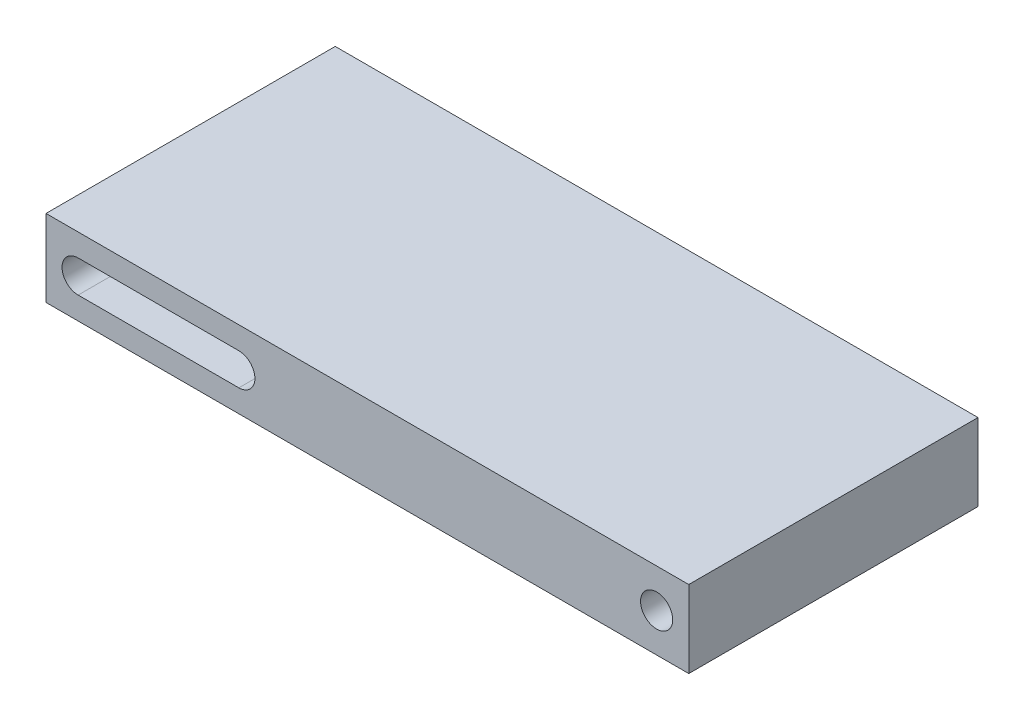
ISO-10303-21;
HEADER;
FILE_DESCRIPTION(('STEP AP214'),'2;1');
FILE_NAME('part.step','',(''),(''),'','','');
FILE_SCHEMA(('AUTOMOTIVE_DESIGN { 1 0 10303 214 1 1 1 1 }'));
ENDSEC;
DATA;
#1=APPLICATION_CONTEXT('core data for automotive mechanical design processes');
#2=APPLICATION_PROTOCOL_DEFINITION('international standard','automotive_design',2000,#1);
#3=PRODUCT_CONTEXT('',#1,'mechanical');
#4=PRODUCT('Part','Part','',(#3));
#5=PRODUCT_RELATED_PRODUCT_CATEGORY('part','',(#4));
#6=PRODUCT_DEFINITION_FORMATION('','',#4);
#7=PRODUCT_DEFINITION_CONTEXT('part definition',#1,'design');
#8=PRODUCT_DEFINITION('design','',#6,#7);
#9=PRODUCT_DEFINITION_SHAPE('','',#8);
#10=(LENGTH_UNIT() NAMED_UNIT(*) SI_UNIT(.MILLI.,.METRE.));
#11=(NAMED_UNIT(*) PLANE_ANGLE_UNIT() SI_UNIT($,.RADIAN.));
#12=(NAMED_UNIT(*) SI_UNIT($,.STERADIAN.) SOLID_ANGLE_UNIT());
#13=UNCERTAINTY_MEASURE_WITH_UNIT(LENGTH_MEASURE(1.E-05),#10,'distance_accuracy_value','');
#14=(GEOMETRIC_REPRESENTATION_CONTEXT(3) GLOBAL_UNCERTAINTY_ASSIGNED_CONTEXT((#13)) GLOBAL_UNIT_ASSIGNED_CONTEXT((#10,
#11,#12)) REPRESENTATION_CONTEXT('',''));
#15=CARTESIAN_POINT('',(0.,0.,0.));
#16=DIRECTION('',(0.,0.,1.));
#17=DIRECTION('',(1.,0.,0.));
#18=AXIS2_PLACEMENT_3D('',#15,#16,#17);
#19=CARTESIAN_POINT('',(50.,6.,22.5));
#20=DIRECTION('',(-1.,0.,0.));
#21=DIRECTION('',(0.,0.,1.));
#22=AXIS2_PLACEMENT_3D('',#19,#20,#21);
#23=PLANE('',#22);
#24=DIRECTION('',(0.,1.,0.));
#25=VECTOR('',#24,1.);
#26=CARTESIAN_POINT('',(50.,6.,-22.5));
#27=LINE('',#26,#25);
#28=CARTESIAN_POINT('',(50.,-6.,-22.5));
#29=VERTEX_POINT('',#28);
#30=CARTESIAN_POINT('',(50.,6.,-22.5));
#31=VERTEX_POINT('',#30);
#32=EDGE_CURVE('E116',#29,#31,#27,.T.);
#33=ORIENTED_EDGE('',*,*,#32,.T.);
#34=DIRECTION('',(0.,0.,-1.));
#35=VECTOR('',#34,1.);
#36=CARTESIAN_POINT('',(50.,6.,22.5));
#37=LINE('',#36,#35);
#38=CARTESIAN_POINT('',(50.,6.,22.5));
#39=VERTEX_POINT('',#38);
#40=EDGE_CURVE('E11',#39,#31,#37,.T.);
#41=ORIENTED_EDGE('',*,*,#40,.F.);
#42=DIRECTION('',(0.,1.,0.));
#43=VECTOR('',#42,1.);
#44=CARTESIAN_POINT('',(50.,6.,22.5));
#45=LINE('',#44,#43);
#46=CARTESIAN_POINT('',(50.,-6.,22.5));
#47=VERTEX_POINT('',#46);
#48=EDGE_CURVE('E148',#47,#39,#45,.T.);
#49=ORIENTED_EDGE('',*,*,#48,.F.);
#50=DIRECTION('',(0.,0.,-1.));
#51=VECTOR('',#50,1.);
#52=CARTESIAN_POINT('',(50.,-6.,22.5));
#53=LINE('',#52,#51);
#54=EDGE_CURVE('E156',#47,#29,#53,.T.);
#55=ORIENTED_EDGE('',*,*,#54,.T.);
#56=EDGE_LOOP('',(#33,#41,#49,#55));
#57=FACE_BOUND('',#56,.T.);
#58=ADVANCED_FACE('F39',(#57),#23,.F.);
#59=CARTESIAN_POINT('',(-50.,6.,22.5));
#60=DIRECTION('',(0.,-1.,0.));
#61=DIRECTION('',(0.,0.,-1.));
#62=AXIS2_PLACEMENT_3D('',#59,#60,#61);
#63=PLANE('',#62);
#64=DIRECTION('',(-1.,0.,0.));
#65=VECTOR('',#64,1.);
#66=CARTESIAN_POINT('',(-50.,6.,-22.5));
#67=LINE('',#66,#65);
#68=CARTESIAN_POINT('',(-50.,6.,-22.5));
#69=VERTEX_POINT('',#68);
#70=EDGE_CURVE('E157',#31,#69,#67,.T.);
#71=ORIENTED_EDGE('',*,*,#70,.T.);
#72=DIRECTION('',(0.,0.,-1.));
#73=VECTOR('',#72,1.);
#74=CARTESIAN_POINT('',(-50.,6.,22.5));
#75=LINE('',#74,#73);
#76=CARTESIAN_POINT('',(-50.,6.,22.5));
#77=VERTEX_POINT('',#76);
#78=EDGE_CURVE('E46',#77,#69,#75,.T.);
#79=ORIENTED_EDGE('',*,*,#78,.F.);
#80=DIRECTION('',(-1.,0.,0.));
#81=VECTOR('',#80,1.);
#82=CARTESIAN_POINT('',(-50.,6.,22.5));
#83=LINE('',#82,#81);
#84=EDGE_CURVE('E149',#39,#77,#83,.T.);
#85=ORIENTED_EDGE('',*,*,#84,.F.);
#86=ORIENTED_EDGE('',*,*,#40,.T.);
#87=EDGE_LOOP('',(#71,#79,#85,#86));
#88=FACE_BOUND('',#87,.T.);
#89=ADVANCED_FACE('F190',(#88),#63,.F.);
#90=CARTESIAN_POINT('',(-50.,6.,22.5));
#91=DIRECTION('',(1.,0.,0.));
#92=DIRECTION('',(0.,0.,-1.));
#93=AXIS2_PLACEMENT_3D('',#90,#91,#92);
#94=PLANE('',#93);
#95=DIRECTION('',(0.,-1.,0.));
#96=VECTOR('',#95,1.);
#97=CARTESIAN_POINT('',(-50.,6.,-22.5));
#98=LINE('',#97,#96);
#99=CARTESIAN_POINT('',(-50.,-6.,-22.5));
#100=VERTEX_POINT('',#99);
#101=EDGE_CURVE('E161',#69,#100,#98,.T.);
#102=ORIENTED_EDGE('',*,*,#101,.T.);
#103=DIRECTION('',(0.,0.,-1.));
#104=VECTOR('',#103,1.);
#105=CARTESIAN_POINT('',(-50.,-6.,22.5));
#106=LINE('',#105,#104);
#107=CARTESIAN_POINT('',(-50.,-6.,22.5));
#108=VERTEX_POINT('',#107);
#109=EDGE_CURVE('E167',#108,#100,#106,.T.);
#110=ORIENTED_EDGE('',*,*,#109,.F.);
#111=DIRECTION('',(0.,-1.,0.));
#112=VECTOR('',#111,1.);
#113=CARTESIAN_POINT('',(-50.,6.,22.5));
#114=LINE('',#113,#112);
#115=EDGE_CURVE('E155',#77,#108,#114,.T.);
#116=ORIENTED_EDGE('',*,*,#115,.F.);
#117=ORIENTED_EDGE('',*,*,#78,.T.);
#118=EDGE_LOOP('',(#102,#110,#116,#117));
#119=FACE_BOUND('',#118,.T.);
#120=ADVANCED_FACE('F175',(#119),#94,.F.);
#121=CARTESIAN_POINT('',(-50.,-6.,22.5));
#122=DIRECTION('',(0.,1.,0.));
#123=DIRECTION('',(0.,0.,1.));
#124=AXIS2_PLACEMENT_3D('',#121,#122,#123);
#125=PLANE('',#124);
#126=DIRECTION('',(1.,0.,0.));
#127=VECTOR('',#126,1.);
#128=CARTESIAN_POINT('',(-50.,-6.,-22.5));
#129=LINE('',#128,#127);
#130=EDGE_CURVE('E147',#100,#29,#129,.T.);
#131=ORIENTED_EDGE('',*,*,#130,.T.);
#132=ORIENTED_EDGE('',*,*,#54,.F.);
#133=DIRECTION('',(1.,0.,0.));
#134=VECTOR('',#133,1.);
#135=CARTESIAN_POINT('',(-50.,-6.,22.5));
#136=LINE('',#135,#134);
#137=EDGE_CURVE('E152',#108,#47,#136,.T.);
#138=ORIENTED_EDGE('',*,*,#137,.F.);
#139=ORIENTED_EDGE('',*,*,#109,.T.);
#140=EDGE_LOOP('',(#131,#132,#138,#139));
#141=FACE_BOUND('',#140,.T.);
#142=ADVANCED_FACE('F182',(#141),#125,.F.);
#143=CARTESIAN_POINT('',(0.,0.,22.5));
#144=DIRECTION('',(0.,0.,1.));
#145=DIRECTION('',(1.,0.,0.));
#146=AXIS2_PLACEMENT_3D('',#143,#144,#145);
#147=PLANE('',#146);
#148=CARTESIAN_POINT('',(-45.,0.,22.5));
#149=DIRECTION('',(0.,0.,1.));
#150=DIRECTION('',(1.,0.,0.));
#151=AXIS2_PLACEMENT_3D('',#148,#149,#150);
#152=CIRCLE('',#151,2.5);
#153=CARTESIAN_POINT('',(-45.,2.5,22.5));
#154=VERTEX_POINT('',#153);
#155=CARTESIAN_POINT('',(-45.,-2.5,22.5));
#156=VERTEX_POINT('',#155);
#157=EDGE_CURVE('E52',#154,#156,#152,.T.);
#158=ORIENTED_EDGE('',*,*,#157,.F.);
#159=DIRECTION('',(-1.,0.,0.));
#160=VECTOR('',#159,1.);
#161=CARTESIAN_POINT('',(-45.,2.5,22.5));
#162=LINE('',#161,#160);
#163=CARTESIAN_POINT('',(-20.,2.5,22.5));
#164=VERTEX_POINT('',#163);
#165=EDGE_CURVE('E112',#164,#154,#162,.T.);
#166=ORIENTED_EDGE('',*,*,#165,.F.);
#167=CARTESIAN_POINT('',(-20.,0.,22.5));
#168=DIRECTION('',(0.,0.,1.));
#169=DIRECTION('',(1.,0.,0.));
#170=AXIS2_PLACEMENT_3D('',#167,#168,#169);
#171=CIRCLE('',#170,2.5);
#172=CARTESIAN_POINT('',(-20.,-2.5,22.5));
#173=VERTEX_POINT('',#172);
#174=EDGE_CURVE('E134',#173,#164,#171,.T.);
#175=ORIENTED_EDGE('',*,*,#174,.F.);
#176=DIRECTION('',(1.,0.,0.));
#177=VECTOR('',#176,1.);
#178=CARTESIAN_POINT('',(-45.,-2.5,22.5));
#179=LINE('',#178,#177);
#180=EDGE_CURVE('E124',#156,#173,#179,.T.);
#181=ORIENTED_EDGE('',*,*,#180,.F.);
#182=EDGE_LOOP('',(#158,#166,#175,#181));
#183=FACE_BOUND('',#182,.T.);
#184=CARTESIAN_POINT('',(45.,0.,22.5));
#185=DIRECTION('',(0.,0.,1.));
#186=DIRECTION('',(1.,0.,0.));
#187=AXIS2_PLACEMENT_3D('',#184,#185,#186);
#188=CIRCLE('',#187,2.5);
#189=CARTESIAN_POINT('',(47.5,0.,22.5));
#190=VERTEX_POINT('',#189);
#191=EDGE_CURVE('E139',#190,#190,#188,.T.);
#192=ORIENTED_EDGE('',*,*,#191,.F.);
#193=EDGE_LOOP('',(#192));
#194=FACE_BOUND('',#193,.T.);
#195=ORIENTED_EDGE('',*,*,#48,.T.);
#196=ORIENTED_EDGE('',*,*,#84,.T.);
#197=ORIENTED_EDGE('',*,*,#115,.T.);
#198=ORIENTED_EDGE('',*,*,#137,.T.);
#199=EDGE_LOOP('',(#195,#196,#197,#198));
#200=FACE_BOUND('',#199,.T.);
#201=ADVANCED_FACE('F186',(#183,#194,#200),#147,.T.);
#202=CARTESIAN_POINT('',(0.,0.,-22.5));
#203=DIRECTION('',(0.,0.,1.));
#204=DIRECTION('',(1.,0.,0.));
#205=AXIS2_PLACEMENT_3D('',#202,#203,#204);
#206=PLANE('',#205);
#207=DIRECTION('',(1.,0.,0.));
#208=VECTOR('',#207,1.);
#209=CARTESIAN_POINT('',(-45.,2.5,-22.5));
#210=LINE('',#209,#208);
#211=CARTESIAN_POINT('',(-45.,2.5,-22.5));
#212=VERTEX_POINT('',#211);
#213=CARTESIAN_POINT('',(-20.,2.5,-22.5));
#214=VERTEX_POINT('',#213);
#215=EDGE_CURVE('E122',#212,#214,#210,.T.);
#216=ORIENTED_EDGE('',*,*,#215,.F.);
#217=CARTESIAN_POINT('',(-45.,0.,-22.5));
#218=DIRECTION('',(0.,0.,1.));
#219=DIRECTION('',(1.,0.,0.));
#220=AXIS2_PLACEMENT_3D('',#217,#218,#219);
#221=CIRCLE('',#220,2.5);
#222=CARTESIAN_POINT('',(-45.,-2.5,-22.5));
#223=VERTEX_POINT('',#222);
#224=EDGE_CURVE('E104',#223,#212,#221,.F.);
#225=ORIENTED_EDGE('',*,*,#224,.F.);
#226=DIRECTION('',(-1.,0.,0.));
#227=VECTOR('',#226,1.);
#228=CARTESIAN_POINT('',(-45.,-2.5,-22.5));
#229=LINE('',#228,#227);
#230=CARTESIAN_POINT('',(-20.,-2.5,-22.5));
#231=VERTEX_POINT('',#230);
#232=EDGE_CURVE('E111',#231,#223,#229,.T.);
#233=ORIENTED_EDGE('',*,*,#232,.F.);
#234=CARTESIAN_POINT('',(-20.,0.,-22.5));
#235=DIRECTION('',(0.,0.,1.));
#236=DIRECTION('',(1.,0.,0.));
#237=AXIS2_PLACEMENT_3D('',#234,#235,#236);
#238=CIRCLE('',#237,2.5);
#239=EDGE_CURVE('E64',#214,#231,#238,.F.);
#240=ORIENTED_EDGE('',*,*,#239,.F.);
#241=EDGE_LOOP('',(#216,#225,#233,#240));
#242=FACE_BOUND('',#241,.T.);
#243=CARTESIAN_POINT('',(45.,0.,-22.5));
#244=DIRECTION('',(0.,0.,1.));
#245=DIRECTION('',(1.,0.,0.));
#246=AXIS2_PLACEMENT_3D('',#243,#244,#245);
#247=CIRCLE('',#246,2.5);
#248=CARTESIAN_POINT('',(47.5,0.,-22.5));
#249=VERTEX_POINT('',#248);
#250=EDGE_CURVE('E141',#249,#249,#247,.F.);
#251=ORIENTED_EDGE('',*,*,#250,.F.);
#252=EDGE_LOOP('',(#251));
#253=FACE_BOUND('',#252,.T.);
#254=ORIENTED_EDGE('',*,*,#32,.F.);
#255=ORIENTED_EDGE('',*,*,#130,.F.);
#256=ORIENTED_EDGE('',*,*,#101,.F.);
#257=ORIENTED_EDGE('',*,*,#70,.F.);
#258=EDGE_LOOP('',(#254,#255,#256,#257));
#259=FACE_BOUND('',#258,.T.);
#260=ADVANCED_FACE('F117',(#242,#253,#259),#206,.F.);
#261=CARTESIAN_POINT('',(45.,0.,-22.501));
#262=DIRECTION('',(0.,0.,1.));
#263=DIRECTION('',(1.,0.,0.));
#264=AXIS2_PLACEMENT_3D('',#261,#262,#263);
#265=CYLINDRICAL_SURFACE('',#264,2.5);
#266=ORIENTED_EDGE('',*,*,#191,.T.);
#267=EDGE_LOOP('',(#266));
#268=FACE_BOUND('',#267,.T.);
#269=ORIENTED_EDGE('',*,*,#250,.T.);
#270=EDGE_LOOP('',(#269));
#271=FACE_BOUND('',#270,.T.);
#272=ADVANCED_FACE('F199',(#268,#271),#265,.F.);
#273=CARTESIAN_POINT('',(-45.,0.,-22.501));
#274=DIRECTION('',(0.,0.,1.));
#275=DIRECTION('',(1.,0.,0.));
#276=AXIS2_PLACEMENT_3D('',#273,#274,#275);
#277=CYLINDRICAL_SURFACE('',#276,2.5);
#278=ORIENTED_EDGE('',*,*,#224,.T.);
#279=DIRECTION('',(0.,0.,1.));
#280=VECTOR('',#279,1.);
#281=CARTESIAN_POINT('',(-45.,2.5,-22.501));
#282=LINE('',#281,#280);
#283=EDGE_CURVE('E120',#212,#154,#282,.T.);
#284=ORIENTED_EDGE('',*,*,#283,.T.);
#285=ORIENTED_EDGE('',*,*,#157,.T.);
#286=DIRECTION('',(0.,0.,1.));
#287=VECTOR('',#286,1.);
#288=CARTESIAN_POINT('',(-45.,-2.5,-22.501));
#289=LINE('',#288,#287);
#290=EDGE_CURVE('E101',#223,#156,#289,.T.);
#291=ORIENTED_EDGE('',*,*,#290,.F.);
#292=EDGE_LOOP('',(#278,#284,#285,#291));
#293=FACE_BOUND('',#292,.T.);
#294=ADVANCED_FACE('F103',(#293),#277,.F.);
#295=CARTESIAN_POINT('',(-45.,2.5,-22.501));
#296=DIRECTION('',(0.,1.,0.));
#297=DIRECTION('',(0.,0.,1.));
#298=AXIS2_PLACEMENT_3D('',#295,#296,#297);
#299=PLANE('',#298);
#300=ORIENTED_EDGE('',*,*,#215,.T.);
#301=DIRECTION('',(0.,0.,1.));
#302=VECTOR('',#301,1.);
#303=CARTESIAN_POINT('',(-20.,2.5,-22.501));
#304=LINE('',#303,#302);
#305=EDGE_CURVE('E140',#214,#164,#304,.T.);
#306=ORIENTED_EDGE('',*,*,#305,.T.);
#307=ORIENTED_EDGE('',*,*,#165,.T.);
#308=ORIENTED_EDGE('',*,*,#283,.F.);
#309=EDGE_LOOP('',(#300,#306,#307,#308));
#310=FACE_BOUND('',#309,.T.);
#311=ADVANCED_FACE('F207',(#310),#299,.F.);
#312=CARTESIAN_POINT('',(-20.,0.,-22.501));
#313=DIRECTION('',(0.,0.,1.));
#314=DIRECTION('',(1.,0.,0.));
#315=AXIS2_PLACEMENT_3D('',#312,#313,#314);
#316=CYLINDRICAL_SURFACE('',#315,2.5);
#317=ORIENTED_EDGE('',*,*,#239,.T.);
#318=DIRECTION('',(0.,0.,1.));
#319=VECTOR('',#318,1.);
#320=CARTESIAN_POINT('',(-20.,-2.5,-22.501));
#321=LINE('',#320,#319);
#322=EDGE_CURVE('E109',#231,#173,#321,.T.);
#323=ORIENTED_EDGE('',*,*,#322,.T.);
#324=ORIENTED_EDGE('',*,*,#174,.T.);
#325=ORIENTED_EDGE('',*,*,#305,.F.);
#326=EDGE_LOOP('',(#317,#323,#324,#325));
#327=FACE_BOUND('',#326,.T.);
#328=ADVANCED_FACE('F215',(#327),#316,.F.);
#329=CARTESIAN_POINT('',(-45.,-2.5,-22.501));
#330=DIRECTION('',(0.,-1.,0.));
#331=DIRECTION('',(0.,0.,-1.));
#332=AXIS2_PLACEMENT_3D('',#329,#330,#331);
#333=PLANE('',#332);
#334=ORIENTED_EDGE('',*,*,#232,.T.);
#335=ORIENTED_EDGE('',*,*,#290,.T.);
#336=ORIENTED_EDGE('',*,*,#180,.T.);
#337=ORIENTED_EDGE('',*,*,#322,.F.);
#338=EDGE_LOOP('',(#334,#335,#336,#337));
#339=FACE_BOUND('',#338,.T.);
#340=ADVANCED_FACE('F113',(#339),#333,.F.);
#341=CLOSED_SHELL('',(#58,#89,#120,#142,#201,#260,#272,#294,#311,#328,#340));
#342=MANIFOLD_SOLID_BREP('B2',#341);
#343=ADVANCED_BREP_SHAPE_REPRESENTATION('',(#18,#342),#14);
#344=SHAPE_DEFINITION_REPRESENTATION(#9,#343);
ENDSEC;
END-ISO-10303-21;
